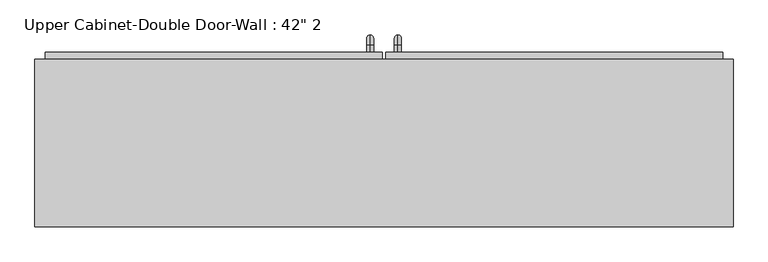
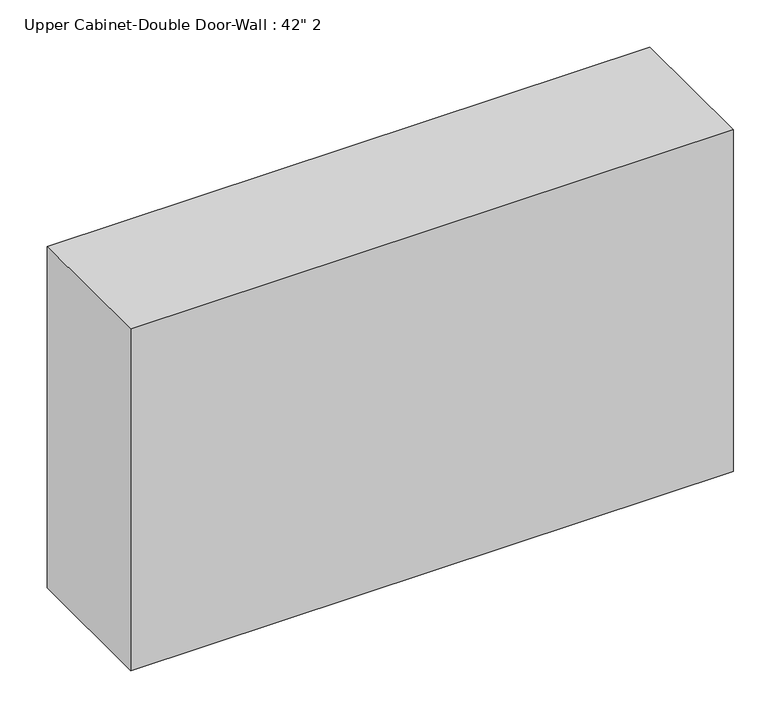
"""IFC4 building model written with IfcOpenShell, lengths in millimetres: furniture geometry."""

from ifc_helpers import new_model, si_unit, point, frame, origin, place, context, project, spatial, polyline, circle_curve, ellipse_curve, trimmed, outline, extrude, faceted_brep, source, transform, mapped, element, save
from ifc_brep_helpers import plane_surface, cylinder_surface, revolved_surface, advanced_brep


def furniture_4a8f7e85(model_context):
    return source(origin(), model_context, "Body", "SolidModel", [
        extrude(outline(polyline([(32.9461628, 374.65), (645.7211628, 374.65), (645.7211628, 342.9), (32.9461628, 342.9), (32.9461628, 374.65)])), frame((0.0, 0.0, 1390.65), z_axis=(0.0, 0.0, 1.0), x_axis=(1.0, 0.0, 0.0)), (0.0, 0.0, 1.0), 723.9),
        extrude(outline(polyline([(-586.1788372, 374.65), (26.5961628, 374.65), (26.5961628, 342.9), (-586.1788372, 342.9), (-586.1788372, 374.65)])), frame((0.0, 0.0, 1390.65), z_axis=(0.0, 0.0, 1.0), x_axis=(1.0, 0.0, 0.0)), (0.0, 0.0, 1.0), 723.9),
        advanced_brep(
        [(4.3711628, 374.65, 1517.65), (4.3711628, 374.65, 1530.35), (4.3711628, 387.35, 1517.65), (4.3711628, 387.35, 1530.35), (4.3711628, 406.4, 1511.3), (4.3711628, 393.7, 1511.3), (4.3711628, 393.7, 1435.1), (4.3711628, 406.4, 1435.1), (4.3711628, 387.35, 1416.05), (4.3711628, 387.35, 1428.75), (4.3711628, 374.65, 1428.75), (4.3711628, 374.65, 1416.05)],
        [
            (0, 1, circle_curve(frame((4.3711628, 374.65, 1524.0), z_axis=(0.0, -1.0, 0.0), x_axis=(0.0, 0.0, 1.0)), 6.35)),
            (1, 0, circle_curve(frame((4.3711628, 374.65, 1524.0), z_axis=(0.0, -1.0, 0.0), x_axis=(0.0, 0.0, 1.0)), 6.35)),
            (0, 2),
            (2, 3, circle_curve(frame((4.3711628, 387.35, 1524.0), z_axis=(0.0, -1.0, 0.0), x_axis=(0.0, 0.0, 1.0)), 6.35)),
            (3, 1),
            (3, 2, circle_curve(frame((4.3711628, 387.35, 1524.0), z_axis=(0.0, -1.0, 0.0), x_axis=(0.0, 0.0, 1.0)), 6.35)),
            (4, 3, circle_curve(frame((4.3711628, 387.35, 1511.3), z_axis=(1.0, 0.0, 0.0), x_axis=(0.0, 0.0, 1.0)), 19.05)),
            (2, 5, circle_curve(frame((4.3711628, 387.35, 1511.3), z_axis=(-1.0, 0.0, 0.0), x_axis=(0.0, 0.0, 1.0)), 6.35)),
            (5, 4, circle_curve(frame((4.3711628, 400.05, 1511.3), z_axis=(0.0, 0.0, 1.0), x_axis=(0.0, 1.0, 0.0)), 6.35)),
            (4, 5, circle_curve(frame((4.3711628, 400.05, 1511.3), z_axis=(0.0, 0.0, 1.0), x_axis=(0.0, 1.0, 0.0)), 6.35)),
            (5, 6),
            (6, 7, circle_curve(frame((4.3711628, 400.05, 1435.1), z_axis=(0.0, 0.0, 1.0), x_axis=(0.0, 1.0, 0.0)), 6.35)),
            (7, 4),
            (7, 6, circle_curve(frame((4.3711628, 400.05, 1435.1), z_axis=(0.0, 0.0, 1.0), x_axis=(0.0, 1.0, 0.0)), 6.35)),
            (8, 7, circle_curve(frame((4.3711628, 387.35, 1435.1), z_axis=(1.0, 0.0, 0.0), x_axis=(0.0, 1.0, 0.0)), 19.05)),
            (6, 9, circle_curve(frame((4.3711628, 387.35, 1435.1), z_axis=(-1.0, 0.0, 0.0), x_axis=(0.0, 1.0, 0.0)), 6.35)),
            (9, 8, circle_curve(frame((4.3711628, 387.35, 1422.4), z_axis=(0.0, 1.0, 0.0), x_axis=(0.0, 0.0, -1.0)), 6.35)),
            (8, 9, circle_curve(frame((4.3711628, 387.35, 1422.4), z_axis=(0.0, 1.0, 0.0), x_axis=(0.0, 0.0, -1.0)), 6.35)),
            (10, 11, circle_curve(frame((4.3711628, 374.65, 1422.4), z_axis=(0.0, -1.0, 0.0), x_axis=(0.0, 0.0, -1.0)), 6.35)),
            (11, 10, circle_curve(frame((4.3711628, 374.65, 1422.4), z_axis=(0.0, -1.0, 0.0), x_axis=(0.0, 0.0, -1.0)), 6.35)),
            (9, 10),
            (11, 8),
        ],
        [
            plane_surface(frame((-1.9788372, 374.65, 1524.0), z_axis=(0.0, -1.0, 0.0), x_axis=(0.0, 0.0, 1.0))),
            cylinder_surface(frame((4.3711628, 374.65, 1524.0), z_axis=(0.0, -1.0, 0.0), x_axis=(0.0, 0.0, 1.0)), 6.35),
            revolved_surface(trimmed(ellipse_curve(frame((4.3711628, 387.35, 1524.0), z_axis=(0.0, -1.0, 0.0), x_axis=(0.0, 0.0, 1.0)), 6.35, 6.35), [point((4.3711628, 387.35, 1517.65))], [point((4.3711628, 387.35, 1530.35))], True, "CARTESIAN"), (4.3711628, 387.35, 1511.3), (-1.0, 0.0, 0.0)),
            revolved_surface(trimmed(ellipse_curve(frame((4.3711628, 387.35, 1524.0), z_axis=(0.0, -1.0, 0.0), x_axis=(0.0, 0.0, 1.0)), 6.35, 6.35), [point((4.3711628, 387.35, 1530.35))], [point((4.3711628, 387.35, 1517.65))], True, "CARTESIAN"), (4.3711628, 387.35, 1511.3), (-1.0, 0.0, 0.0)),
            cylinder_surface(frame((4.3711628, 400.05, 1511.3), z_axis=(0.0, 0.0, 1.0), x_axis=(0.0, 1.0, 0.0)), 6.35),
            revolved_surface(trimmed(ellipse_curve(frame((4.3711628, 400.05, 1435.1), z_axis=(0.0, 0.0, 1.0), x_axis=(0.0, 1.0, 0.0)), 6.35, 6.35), [point((4.3711628, 393.7, 1435.1))], [point((4.3711628, 406.4, 1435.1))], True, "CARTESIAN"), (4.3711628, 387.35, 1435.1), (-1.0, 0.0, 0.0)),
            revolved_surface(trimmed(ellipse_curve(frame((4.3711628, 400.05, 1435.1), z_axis=(0.0, 0.0, 1.0), x_axis=(0.0, 1.0, 0.0)), 6.35, 6.35), [point((4.3711628, 406.4, 1435.1))], [point((4.3711628, 393.7, 1435.1))], True, "CARTESIAN"), (4.3711628, 387.35, 1435.1), (-1.0, 0.0, 0.0)),
            plane_surface(frame((-1.9788372, 374.65, 1422.4), z_axis=(0.0, -1.0, 0.0), x_axis=(0.0, 0.0, -1.0))),
            cylinder_surface(frame((4.3711628, 387.35, 1422.4), z_axis=(0.0, 1.0, 0.0), x_axis=(0.0, 0.0, -1.0)), 6.35),
        ],
        [
            (0, [[1, 2]]),
            (1, [[-1, 3, 4, 5]]),
            (1, [[-2, -5, 6, -3]]),
            (2, [[7, -4, 8, 9]]),
            (3, [[-8, -6, -7, 10]]),
            (4, [[-9, 11, 12, 13]]),
            (4, [[-10, -13, 14, -11]]),
            (5, [[15, -12, 16, 17]]),
            (6, [[-16, -14, -15, 18]]),
            (7, [[19, 20]]),
            (8, [[-17, 21, -20, 22]]),
            (8, [[-18, -22, -19, -21]]),
        ],
    ),
        advanced_brep(
        [(55.1711628, 374.65, 1517.65), (55.1711628, 374.65, 1530.35), (55.1711628, 387.35, 1517.65), (55.1711628, 387.35, 1530.35), (55.1711628, 406.4, 1511.3), (55.1711628, 393.7, 1511.3), (55.1711628, 393.7, 1435.1), (55.1711628, 406.4, 1435.1), (55.1711628, 387.35, 1416.05), (55.1711628, 387.35, 1428.75), (55.1711628, 374.65, 1428.75), (55.1711628, 374.65, 1416.05)],
        [
            (0, 1, circle_curve(frame((55.1711628, 374.65, 1524.0), z_axis=(0.0, -1.0, 0.0), x_axis=(0.0, 0.0, -1.0)), 6.35)),
            (1, 0, circle_curve(frame((55.1711628, 374.65, 1524.0), z_axis=(0.0, -1.0, 0.0), x_axis=(0.0, 0.0, -1.0)), 6.35)),
            (0, 2),
            (2, 3, circle_curve(frame((55.1711628, 387.35, 1524.0), z_axis=(0.0, -1.0, 0.0), x_axis=(0.0, 0.0, -1.0)), 6.35)),
            (3, 1),
            (3, 2, circle_curve(frame((55.1711628, 387.35, 1524.0), z_axis=(0.0, -1.0, 0.0), x_axis=(0.0, 0.0, -1.0)), 6.35)),
            (4, 3, circle_curve(frame((55.1711628, 387.35, 1511.3), z_axis=(1.0, 0.0, 0.0), x_axis=(0.0, 0.0, 1.0)), 19.05)),
            (2, 5, circle_curve(frame((55.1711628, 387.35, 1511.3), z_axis=(-1.0, 0.0, 0.0), x_axis=(0.0, 0.0, 1.0)), 6.35)),
            (5, 4, circle_curve(frame((55.1711628, 400.05, 1511.3), z_axis=(0.0, 0.0, 1.0), x_axis=(0.0, -1.0, 0.0)), 6.35)),
            (4, 5, circle_curve(frame((55.1711628, 400.05, 1511.3), z_axis=(0.0, 0.0, 1.0), x_axis=(0.0, -1.0, 0.0)), 6.35)),
            (5, 6),
            (6, 7, circle_curve(frame((55.1711628, 400.05, 1435.1), z_axis=(0.0, 0.0, 1.0), x_axis=(0.0, -1.0, 0.0)), 6.35)),
            (7, 4),
            (7, 6, circle_curve(frame((55.1711628, 400.05, 1435.1), z_axis=(0.0, 0.0, 1.0), x_axis=(0.0, -1.0, 0.0)), 6.35)),
            (8, 7, circle_curve(frame((55.1711628, 387.35, 1435.1), z_axis=(1.0, 0.0, 0.0), x_axis=(0.0, 1.0, 0.0)), 19.05)),
            (6, 9, circle_curve(frame((55.1711628, 387.35, 1435.1), z_axis=(-1.0, 0.0, 0.0), x_axis=(0.0, 1.0, 0.0)), 6.35)),
            (9, 8, circle_curve(frame((55.1711628, 387.35, 1422.4), z_axis=(0.0, 1.0, 0.0), x_axis=(0.0, 0.0, 1.0)), 6.35)),
            (8, 9, circle_curve(frame((55.1711628, 387.35, 1422.4), z_axis=(0.0, 1.0, 0.0), x_axis=(0.0, 0.0, 1.0)), 6.35)),
            (10, 11, circle_curve(frame((55.1711628, 374.65, 1422.4), z_axis=(0.0, -1.0, 0.0), x_axis=(0.0, 0.0, 1.0)), 6.35)),
            (11, 10, circle_curve(frame((55.1711628, 374.65, 1422.4), z_axis=(0.0, -1.0, 0.0), x_axis=(0.0, 0.0, 1.0)), 6.35)),
            (9, 10),
            (11, 8),
        ],
        [
            plane_surface(frame((48.8211628, 374.65, 1524.0), z_axis=(0.0, -1.0, 0.0), x_axis=(0.0, 0.0, 1.0))),
            cylinder_surface(frame((55.1711628, 374.65, 1524.0), z_axis=(0.0, -1.0, 0.0), x_axis=(0.0, 0.0, -1.0)), 6.35),
            revolved_surface(trimmed(ellipse_curve(frame((55.1711628, 387.35, 1524.0), z_axis=(0.0, -1.0, 0.0), x_axis=(0.0, 0.0, -1.0)), 6.35, 6.35), [point((55.1711628, 387.35, 1517.65))], [point((55.1711628, 387.35, 1530.35))], True, "CARTESIAN"), (55.1711628, 387.35, 1511.3), (-1.0, 0.0, 0.0)),
            revolved_surface(trimmed(ellipse_curve(frame((55.1711628, 387.35, 1524.0), z_axis=(0.0, -1.0, 0.0), x_axis=(0.0, 0.0, -1.0)), 6.35, 6.35), [point((55.1711628, 387.35, 1530.35))], [point((55.1711628, 387.35, 1517.65))], True, "CARTESIAN"), (55.1711628, 387.35, 1511.3), (-1.0, 0.0, 0.0)),
            cylinder_surface(frame((55.1711628, 400.05, 1511.3), z_axis=(0.0, 0.0, 1.0), x_axis=(0.0, -1.0, 0.0)), 6.35),
            revolved_surface(trimmed(ellipse_curve(frame((55.1711628, 400.05, 1435.1), z_axis=(0.0, 0.0, 1.0), x_axis=(0.0, -1.0, 0.0)), 6.35, 6.35), [point((55.1711628, 393.7, 1435.1))], [point((55.1711628, 406.4, 1435.1))], True, "CARTESIAN"), (55.1711628, 387.35, 1435.1), (-1.0, 0.0, 0.0)),
            revolved_surface(trimmed(ellipse_curve(frame((55.1711628, 400.05, 1435.1), z_axis=(0.0, 0.0, 1.0), x_axis=(0.0, -1.0, 0.0)), 6.35, 6.35), [point((55.1711628, 406.4, 1435.1))], [point((55.1711628, 393.7, 1435.1))], True, "CARTESIAN"), (55.1711628, 387.35, 1435.1), (-1.0, 0.0, 0.0)),
            plane_surface(frame((48.8211628, 374.65, 1422.4), z_axis=(0.0, -1.0, 0.0), x_axis=(0.0, 0.0, -1.0))),
            cylinder_surface(frame((55.1711628, 387.35, 1422.4), z_axis=(0.0, 1.0, 0.0), x_axis=(0.0, 0.0, 1.0)), 6.35),
        ],
        [
            (0, [[1, 2]]),
            (1, [[-1, 3, 4, 5]]),
            (1, [[-2, -5, 6, -3]]),
            (2, [[7, -4, 8, 9]]),
            (3, [[-8, -6, -7, 10]]),
            (4, [[-9, 11, 12, 13]]),
            (4, [[-10, -13, 14, -11]]),
            (5, [[15, -12, 16, 17]]),
            (6, [[-16, -14, -15, 18]]),
            (7, [[19, 20]]),
            (8, [[-17, 21, -20, 22]]),
            (8, [[-18, -22, -19, -21]]),
        ],
    ),
        faceted_brep([(-605.2288372, 57.15, 2133.6), (-605.2288372, 57.15, 1371.6), (664.7711628, 57.15, 1371.6), (664.7711628, 57.15, 2133.6), (-605.2288372, 361.95, 2133.6), (664.7711628, 361.95, 2133.6), (664.7711628, 361.95, 1371.6), (-605.2288372, 361.95, 1371.6), (-586.1788372, 361.95, 2114.55), (-586.1788372, 361.95, 1390.65), (645.7211628, 361.95, 1390.65), (645.7211628, 361.95, 2114.55), (645.7211628, 76.2, 2114.55), (-586.1788372, 76.2, 2114.55), (645.7211628, 76.2, 1390.65), (-586.1788372, 76.2, 1390.65)], [[[0, 1, 2, 3]], [[4, 5, 6, 7], [8, 9, 10, 11]], [[1, 0, 4, 7]], [[2, 1, 7, 6]], [[3, 2, 6, 5]], [[0, 3, 5, 4]], [[8, 11, 12, 13]], [[11, 10, 14, 12]], [[10, 9, 15, 14]], [[9, 8, 13, 15]], [[13, 12, 14, 15]]]),
    ])


if __name__ == "__main__":
    model = new_model("IFC4")
    model_context = context("Model", 3, world=origin())
    ifc_project = project(units=[si_unit("LENGTHUNIT", "METRE", prefix="MILLI")], contexts=[model_context])
    site = spatial("IfcSite", under=ifc_project)
    building = spatial("IfcBuilding", under=site)
    placement = place(None, origin())
    furniture_shape = furniture_4a8f7e85(model_context)
    element("IfcFurniture", 1, ObjectType="Upper Cabinet-Double Door-Wall : 42\" 2", at=placement, inside=building, context=model_context, shape_type="MappedRepresentation", body=[
        mapped(furniture_shape, transform((0.0, 0.0, 0.0), x_axis=(1.0, 0.0, 0.0), y_axis=(0.0, 1.0, 0.0), z_axis=(0.0, 0.0, 1.0))),
    ])
    save(model, "model.ifc")

# Revit data of these elements
# Type "Upper Cabinet-Double Door-Wall : 42\" 2"
#   Assembly Code = "C1030410"
#   Depth = 1' - 0"
#   Height = 2' - 6"
#   Top Of Cabinet = 7' - 0"
#   Width = 4' - 2"
#   Cabinet Material = none
#   Door/Drawer Material = none
#   Handle Material = Cabinets - Handles
#   Default Elevation = 0
# Element 1 (IfcFurniture, "Upper Cabinet-Double Door-Wall : 42\" 2")
#   Materials on its faces: "Cabinets - Handles", "Cabinet"
# Materials
#   "Cabinets - Handles": colour RGB 57 57 57, transparency 0
#   "Cabinet": colour RGB 204 122 2, transparency 0
